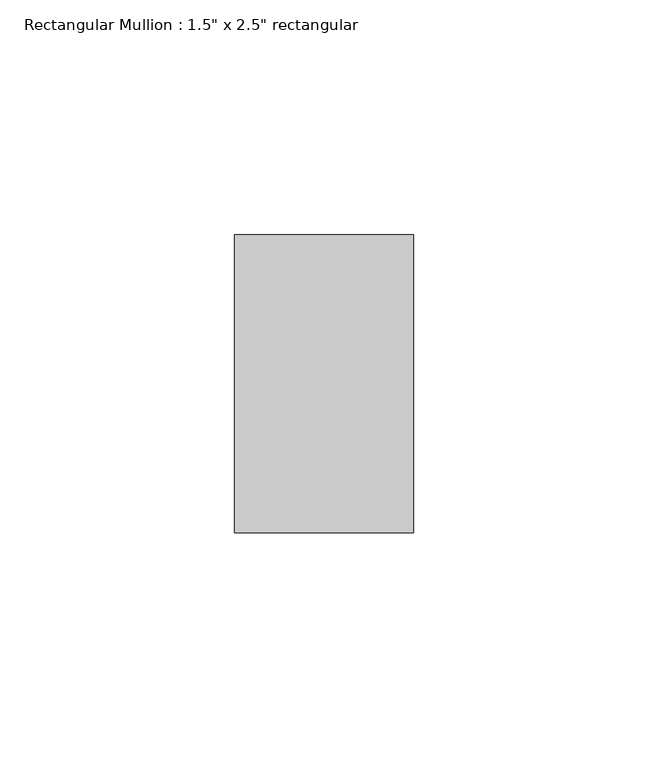
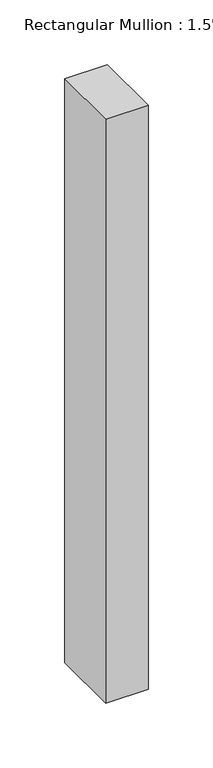
"""IFC4 building model written with IfcOpenShell, lengths in millimetres: member geometry."""

from ifc_helpers import new_model, si_unit, frame, origin, place, context, project, spatial, polyline, outline, extrude, source, transform, mapped, element, save


def member_fa69921b(model_context):
    return source(origin(), model_context, "Body", "SweptSolid", [
        extrude(outline(polyline([(0.0, 31.75), (0.0, -31.75), (-38.1, -31.75), (-38.1, 31.75), (0.0, 31.75)])), frame((0.0, 0.0, -552.4500003), z_axis=(0.0, 0.0, 1.0), x_axis=(1.0, 0.0, 0.0)), (0.0, 0.0, 1.0), 552.4500003),
    ])


if __name__ == "__main__":
    model = new_model("IFC4")
    model_context = context("Model", 3, world=origin())
    ifc_project = project(units=[si_unit("LENGTHUNIT", "METRE", prefix="MILLI")], contexts=[model_context])
    site = spatial("IfcSite", under=ifc_project)
    building = spatial("IfcBuilding", under=site)
    placement = place(None, origin())
    member_shape = member_fa69921b(model_context)
    element("IfcMember", 1, ObjectType="Rectangular Mullion : 1.5\" x 2.5\" rectangular", at=placement, inside=building, context=model_context, shape_type="MappedRepresentation", body=[
        mapped(member_shape, transform((0.0, 0.0, 0.0), x_axis=(1.0, 0.0, 0.0), y_axis=(0.0, 1.0, 0.0), z_axis=(0.0, 0.0, 1.0))),
    ])
    save(model, "model.ifc")

# Revit data of these elements
# Type "Rectangular Mullion : 1.5\" x 2.5\" rectangular"
#   built-in parameter 1007304 = 0.208333 (stored number, unit not read)
#   built-in parameter 1007301 = 0.0625 (stored number, unit not read)
#   built-in parameter 1007300 = 0.0625 (stored number, unit not read)
# Element 1 (IfcMember, "Rectangular Mullion : 1.5\" x 2.5\" rectangular")
#   Materials on its faces: "Aluminum"
# Materials
#   "Aluminum": class "Metal", colour RGB 247 247 247, transparency 0, Description = "Aluminum 6061", Cost = 0
